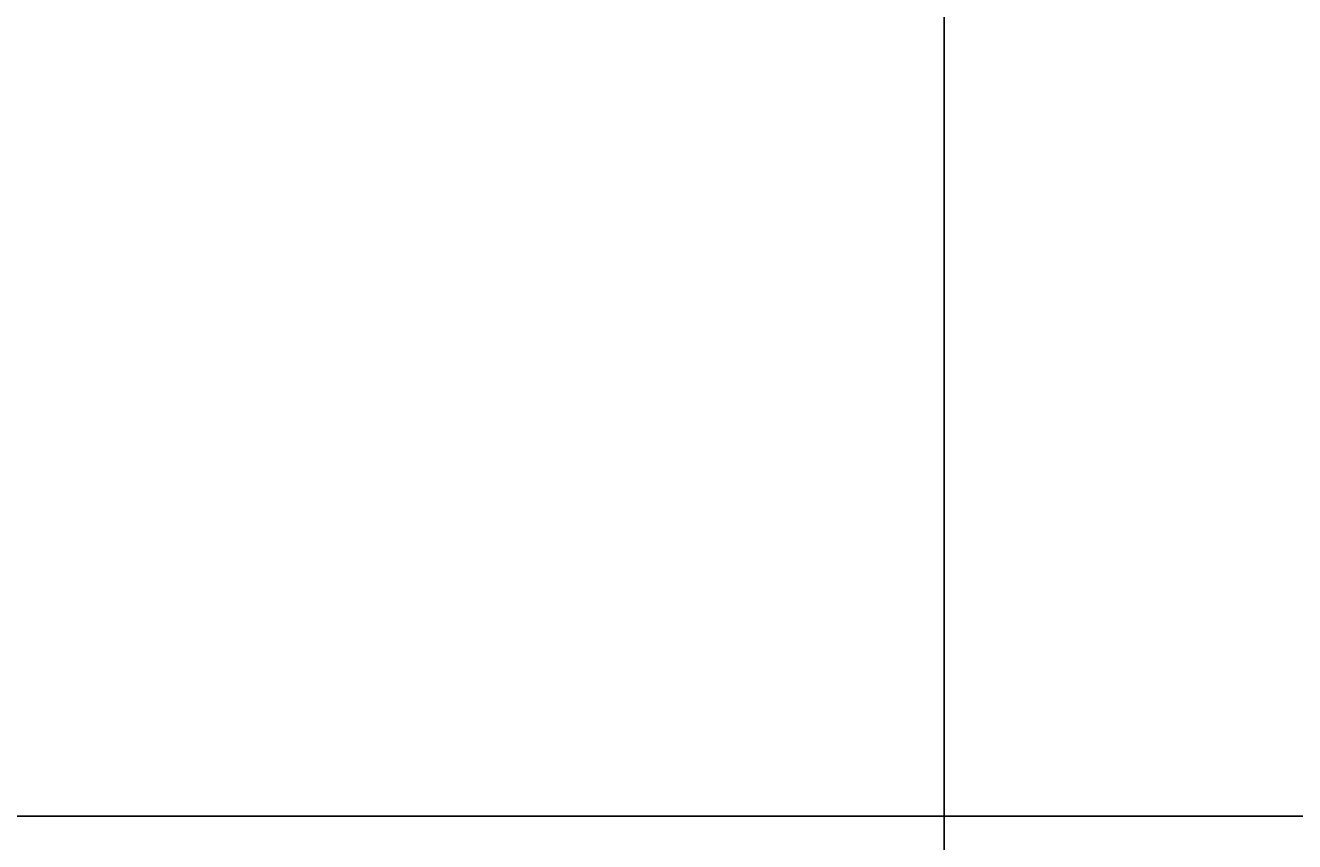
# Model space of a CAD drawing. Units: inches. Extents: x 35362 to 73946, y 43607 to 67532.
# Tile 113 of 134: x 50977 to 51049, y 48969 to 49015. Entities that reach past the tile are written whole.
import ezdxf

# ---------------------------------------------------------------- set-up
doc = ezdxf.new("R2010")
doc.units = ezdxf.units.IN
doc.header["$MEASUREMENT"] = 0
doc.layers.add('A-ANNO-DIMS', color=2, linetype='Continuous', lineweight=18)
doc.styles.get("Standard").update_dxf_attribs({"font": 'arial.ttf'})
doc.dimstyles.get("Standard").update_dxf_attribs({"dimtxt": 0.18, "dimasz": 0.18, "dimexe": 0.18, "dimexo": 0.0625, "dimgap": 0.09, "dimtad": 0, "dimtih": 1, "dimtoh": 1, "dimdec": 4, "dimzin": 0, "dimdsep": 46, "dimtxsty": 'Standard', "dimcen": 0.09, "dimadec": 0, "dimazin": 0, "dimtfac": 1, "dimtdec": 4, "dimtofl": 0, "dimtmove": 0, "dimatfit": 3, "dimfxl": 1, "dimtolj": 1, "dimtzin": 0, "dimarcsym": 0})

# ---------------------------------------------------------------- blocks, each defined once
blk = doc.blocks.new('*D11')
at = {"layer": 'A-ANNO-DIMS', "color": 0, "lineweight": -2, "transparency": 16777216}
for p, q in [((47978.665, 56028.774), (47978.665, 43606.679)), ((53109.76, 56028.774), (53109.76, 43606.679)), ((47978.845, 43606.859), (50543.871, 43606.859)), ((53109.58, 43606.859), (50544.554, 43606.859))]:
    blk.add_line(p, q, dxfattribs=at)
at = {"layer": 'A-ANNO-DIMS', "color": 0, "transparency": 16777216}
for points in [[(47978.845, 43606.889), (47978.845, 43606.829), (47978.665, 43606.859)], [(53109.58, 43606.889), (53109.58, 43606.829), (53109.76, 43606.859)]]:
    blk.add_solid(points, dxfattribs=at)
at = {"layer": 'Defpoints', "color": 0, "transparency": 16777216}
for p in [(47978.665, 56028.836), (53109.76, 56028.836), (53109.76, 43606.859)]:
    blk.add_point(p, dxfattribs=at)
at = {"layer": 'A-ANNO-DIMS', "color": 0, "transparency": 16777216, "insert": (50544.212, 43606.859), "char_height": 0.18, "attachment_point": 5}
blk.add_mtext('\\A1;5131', dxfattribs=at)
blk = doc.blocks.new('*D13')
at = {"layer": 'A-ANNO-DIMS', "color": 0, "lineweight": -2, "transparency": 16777216}
for p, q in [((48373.492, 51694.025), (48373.492, 43606.679)), ((51029.043, 51694.025), (51029.043, 43606.679)), ((48373.672, 43606.859), (49700.802, 43606.859)), ((51028.863, 43606.859), (49701.733, 43606.859))]:
    blk.add_line(p, q, dxfattribs=at)
at = {"layer": 'A-ANNO-DIMS', "color": 0, "transparency": 16777216}
for points in [[(48373.672, 43606.889), (48373.672, 43606.829), (48373.492, 43606.859)], [(51028.863, 43606.889), (51028.863, 43606.829), (51029.043, 43606.859)]]:
    blk.add_solid(points, dxfattribs=at)
at = {"layer": 'Defpoints', "color": 0, "transparency": 16777216}
for p in [(48373.492, 51694.087), (51029.043, 51694.087), (51029.043, 43606.859)]:
    blk.add_point(p, dxfattribs=at)
at = {"layer": 'A-ANNO-DIMS', "color": 0, "transparency": 16777216, "insert": (49701.267, 43606.859), "char_height": 0.18, "attachment_point": 5}
blk.add_mtext('\\A1;2655.6', dxfattribs=at)
blk = doc.blocks.new('*D17')
at = {"layer": 'A-ANNO-DIMS', "color": 0, "lineweight": -2, "transparency": 16777216}
for p, q in [((49923.307, 61293.224), (49923.307, 43606.679)), ((51913.931, 61293.224), (51913.931, 43606.679)), ((49923.487, 43606.859), (50918.164, 43606.859)), ((51913.751, 43606.859), (50919.074, 43606.859))]:
    blk.add_line(p, q, dxfattribs=at)
at = {"layer": 'A-ANNO-DIMS', "color": 0, "transparency": 16777216}
for points in [[(49923.487, 43606.889), (49923.487, 43606.829), (49923.307, 43606.859)], [(51913.751, 43606.889), (51913.751, 43606.829), (51913.931, 43606.859)]]:
    blk.add_solid(points, dxfattribs=at)
at = {"layer": 'Defpoints', "color": 0, "transparency": 16777216}
for p in [(49923.307, 61293.286), (51913.931, 61293.286), (51913.931, 43606.859)]:
    blk.add_point(p, dxfattribs=at)
at = {"layer": 'A-ANNO-DIMS', "color": 0, "transparency": 16777216, "insert": (50918.619, 43606.859), "char_height": 0.18, "attachment_point": 5}
blk.add_mtext('\\A1;1990.6', dxfattribs=at)
blk = doc.blocks.new('*D67')
at = {"layer": 'A-ANNO-DIMS', "color": 0, "lineweight": -2, "transparency": 16777216}
for p, q in [((56873.539, 53351.529), (35361.769, 53351.529)), ((35361.949, 53351.349), (35361.949, 49400.893)), ((35361.949, 45450.074), (35361.949, 49400.53)), ((53793.575, 45449.894), (35361.769, 45449.894))]:
    blk.add_line(p, q, dxfattribs=at)
at = {"layer": 'A-ANNO-DIMS', "color": 0, "transparency": 16777216}
for points in [[(35361.919, 53351.349), (35361.979, 53351.349), (35361.949, 53351.529)], [(35361.919, 45450.074), (35361.979, 45450.074), (35361.949, 45449.894)]]:
    blk.add_solid(points, dxfattribs=at)
at = {"layer": 'Defpoints', "color": 0, "transparency": 16777216}
for p in [(35361.949, 53351.529), (56873.602, 53351.529), (53793.638, 45449.894)]:
    blk.add_point(p, dxfattribs=at)
at = {"layer": 'A-ANNO-DIMS', "color": 0, "transparency": 16777216, "insert": (35361.949, 49400.712), "char_height": 0.18, "attachment_point": 5}
blk.add_mtext('\\A1;7901.6', dxfattribs=at)
blk = doc.blocks.new('*D84')
at = {"layer": 'A-ANNO-DIMS', "color": 0, "lineweight": -2, "transparency": 16777216}
for p, q in [((55540.235, 49259.935), (35361.769, 49259.935)), ((35361.949, 49259.755), (35361.949, 49115.139)), ((35361.949, 48970.16), (35361.949, 49114.776)), ((55540.235, 48969.98), (35361.769, 48969.98))]:
    blk.add_line(p, q, dxfattribs=at)
at = {"layer": 'A-ANNO-DIMS', "color": 0, "transparency": 16777216}
for points in [[(35361.919, 49259.755), (35361.979, 49259.755), (35361.949, 49259.935)], [(35361.919, 48970.16), (35361.979, 48970.16), (35361.949, 48969.98)]]:
    blk.add_solid(points, dxfattribs=at)
at = {"layer": 'Defpoints', "color": 0, "transparency": 16777216}
for p in [(35361.949, 49259.935), (55540.297, 49259.935), (55540.297, 48969.98)]:
    blk.add_point(p, dxfattribs=at)
at = {"layer": 'A-ANNO-DIMS', "color": 0, "transparency": 16777216, "insert": (35361.949, 49114.957), "char_height": 0.18, "attachment_point": 5}
blk.add_mtext('\\A1;289.96', dxfattribs=at)
blk = doc.blocks.new('*D86')
at = {"layer": 'A-ANNO-DIMS', "color": 0, "lineweight": -2, "transparency": 16777216}
for p, q in [((51285.532, 49320.079), (35361.769, 49320.079)), ((35361.949, 49319.899), (35361.949, 49120.261)), ((35361.949, 48920.259), (35361.949, 49119.897)), ((51285.532, 48920.079), (35361.769, 48920.079))]:
    blk.add_line(p, q, dxfattribs=at)
at = {"layer": 'A-ANNO-DIMS', "color": 0, "transparency": 16777216}
for points in [[(35361.919, 49319.899), (35361.979, 49319.899), (35361.949, 49320.079)], [(35361.919, 48920.259), (35361.979, 48920.259), (35361.949, 48920.079)]]:
    blk.add_solid(points, dxfattribs=at)
at = {"layer": 'Defpoints', "color": 0, "transparency": 16777216}
for p in [(35361.949, 49320.079), (51285.595, 49320.079), (51285.595, 48920.079)]:
    blk.add_point(p, dxfattribs=at)
at = {"layer": 'A-ANNO-DIMS', "color": 0, "transparency": 16777216, "insert": (35361.949, 49120.079), "char_height": 0.18, "attachment_point": 5}
blk.add_mtext('\\A1;400.0', dxfattribs=at)
blk = doc.blocks.new('*D107')
at = {"layer": 'A-ANNO-DIMS', "color": 0, "lineweight": -2, "transparency": 16777216}
for p, q in [((50139.563, 59850.014), (50139.563, 43606.679)), ((51320.813, 59850.014), (51320.813, 43606.679)), ((50139.743, 43606.859), (50729.733, 43606.859)), ((51320.633, 43606.859), (50730.643, 43606.859))]:
    blk.add_line(p, q, dxfattribs=at)
at = {"layer": 'A-ANNO-DIMS', "color": 0, "transparency": 16777216}
for points in [[(50139.743, 43606.889), (50139.743, 43606.829), (50139.563, 43606.859)], [(51320.633, 43606.889), (51320.633, 43606.829), (51320.813, 43606.859)]]:
    blk.add_solid(points, dxfattribs=at)
at = {"layer": 'Defpoints', "color": 0, "transparency": 16777216}
for p in [(50139.563, 59850.077), (51320.813, 59850.077), (51320.813, 43606.859)]:
    blk.add_point(p, dxfattribs=at)
at = {"layer": 'A-ANNO-DIMS', "color": 0, "transparency": 16777216, "insert": (50730.188, 43606.859), "char_height": 0.18, "attachment_point": 5}
blk.add_mtext('\\A1;1181.3', dxfattribs=at)

msp = doc.modelspace()

# ---------------------------------------------------------------- dimensions: what is measured, and where the dimension line sits
at = {"layer": 'A-ANNO-DIMS'}
for base, p1, p2, override, picture, middle in [((51913.931, 43606.859), (49923.307, 61293.286), (51913.931, 61293.286), {"dimdec": 1, "dimlfac": 1, "dimrnd": 0, "dimzin": 0, "dimdsep": 46, "dimlunit": 2}, '*D17', (50918.619, 43606.859)), ((51320.8133, 43606.859), (50139.5627, 59850.0769), (51320.8133, 59850.0769), {"dimdec": 1, "dimlfac": 1, "dimrnd": 0, "dimzin": 0, "dimdsep": 46, "dimlunit": 2}, '*D107', (50730.188, 43606.859)), ((53109.76, 43606.859), (47978.665, 56028.836), (53109.76, 56028.836), {"dimdec": 0, "dimlfac": 1, "dimrnd": 0, "dimzin": 0, "dimdsep": 46, "dimlunit": 2}, '*D11', (50544.212, 43606.859)), ((51029.043, 43606.859), (48373.492, 51694.087), (51029.043, 51694.087), {"dimdec": 1, "dimlfac": 1, "dimrnd": 0, "dimzin": 0, "dimdsep": 46, "dimlunit": 2}, '*D13', (49701.267, 43606.859))]:
    dim = msp.add_linear_dim(base=base, p1=p1, p2=p2, dimstyle='Standard', override=override, dxfattribs=at)
    dim.commit()
    dim.dimension.update_dxf_attribs({"geometry": picture, "text_midpoint": middle})
for base, p1, p2, override, picture, middle in [((35361.949, 53351.529), (53793.638, 45449.894), (56873.602, 53351.529), {"dimdec": 1, "dimlfac": 1, "dimrnd": 0, "dimzin": 0, "dimdsep": 46, "dimlunit": 2}, '*D67', (35361.949, 49400.712)), ((35361.949, 49320.079), (51285.595, 48920.079), (51285.595, 49320.079), {"dimdec": 1, "dimlfac": 1, "dimrnd": 0, "dimzin": 0, "dimdsep": 46, "dimlunit": 2}, '*D86', (35361.949, 49120.079)), ((35361.9491, 49259.9353), (55540.2972, 48969.9796), (55540.2972, 49259.9353), {"dimdec": 2, "dimlfac": 1, "dimrnd": 0, "dimzin": 0, "dimdsep": 46, "dimlunit": 2}, '*D84', (35361.9491, 49114.9575))]:
    dim = msp.add_linear_dim(base=base, p1=p1, p2=p2, angle=90, dimstyle='Standard', override=override, dxfattribs=at)
    dim.commit()
    dim.dimension.update_dxf_attribs({"geometry": picture, "text_midpoint": middle})

doc.saveas('drawing.dxf')
